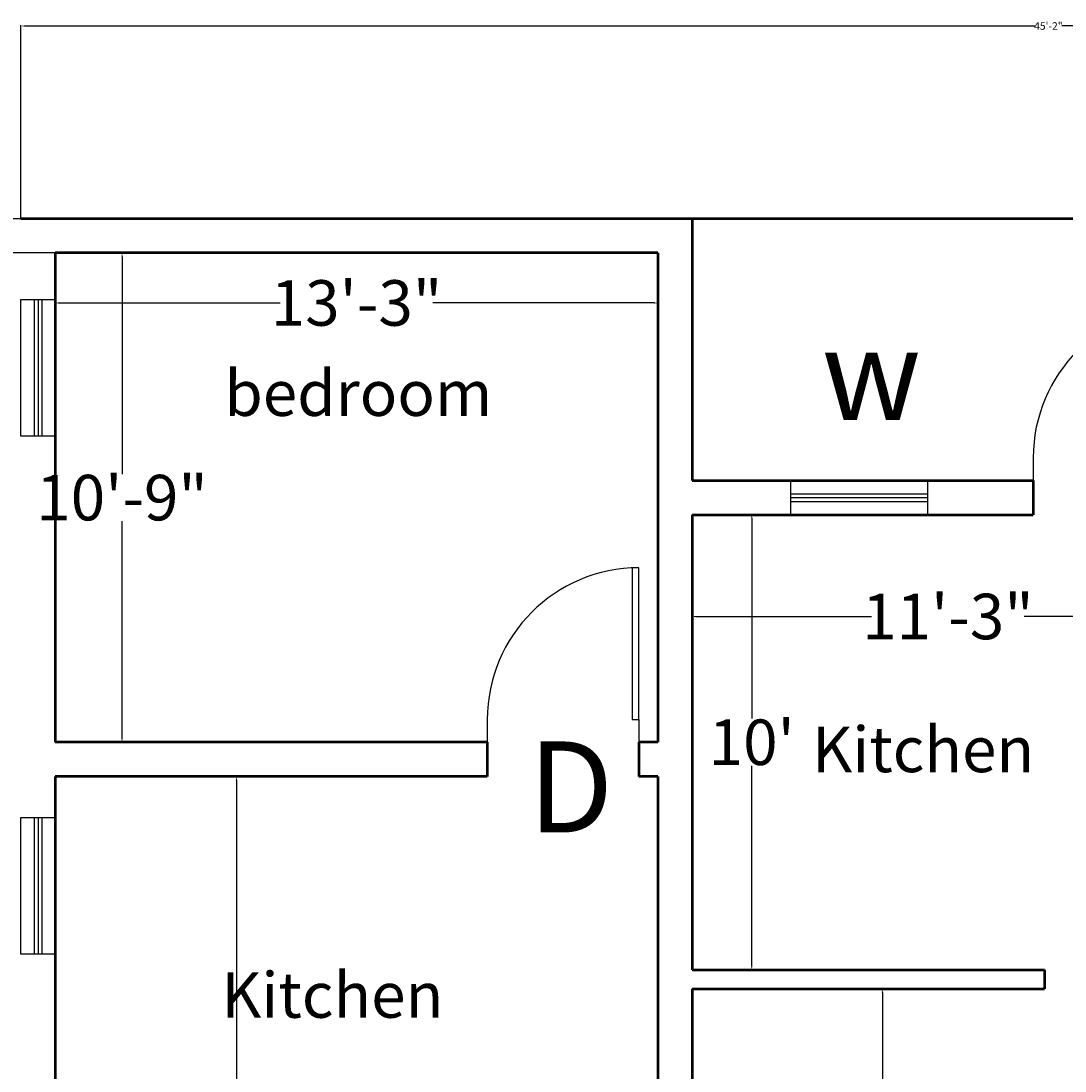
# Model space of a CAD drawing. Units: inches. Extents: x 409 to 7572, y 7 to 725.
# Tile 30 of 38: x 5677 to 5952, y 448 to 725. Entities that reach past the tile are written whole.
import ezdxf

# ---------------------------------------------------------------- set-up
doc = ezdxf.new("R2010")
doc.units = ezdxf.units.IN
doc.header["$MEASUREMENT"] = 0
for name, color, linetype, lineweight in [('A-ANNO-DIMS', 2, 'Continuous', 18), ('A-ANNO-SYMB', 3, 'Continuous', 25), ('A-AREA-IDEN', 7, 'Continuous', 25), ('A-DOOR', 3, 'Continuous', 25), ('A-GLAZ', 4, 'Continuous', 25), ('A-WALL', 7, 'Continuous', 50)]:
    doc.layers.add(name, color=color, linetype=linetype, lineweight=lineweight)
doc.styles.get("Standard").update_dxf_attribs({"font": 'arial.ttf'})
doc.dimstyles.get("Standard").update_dxf_attribs({"dimtxt": 2, "dimasz": 1, "dimexe": 0.18, "dimexo": 0.0625, "dimgap": 0.09, "dimtad": 0, "dimtih": 1, "dimtoh": 1, "dimdec": 0, "dimzin": 0, "dimdsep": 46, "dimlunit": 3, "dimtxsty": 'Standard', "dimcen": 0.09, "dimadec": 0, "dimazin": 0, "dimtfac": 1, "dimtdec": 0, "dimtofl": 0, "dimtmove": 0, "dimatfit": 3, "dimfxl": 1, "dimtolj": 1, "dimtzin": 0, "dimarcsym": 0})

# ---------------------------------------------------------------- blocks, each defined once
blk = doc.blocks.new('*U2')
for p, q in [((0, 0), (0, -6)), ((-40, 0), (-40, -6))]:
    blk.add_line(p, q)
blk.add_lwpolyline([(0, 0), (0, 40), (-1.75, 40), (-1.75, 0)], close=True)
blk.add_arc((0, 0), 40, 90, 180)
blk = doc.blocks.new('*D127')
at = {"layer": 'A-ANNO-DIMS', "color": 0, "lineweight": -2, "transparency": 16777216}
for p, q in [((5685.85, 663.53), (5703.62, 663.53)), ((5703.44, 662.53), (5703.44, 605.25)), ((5703.44, 535.53), (5703.44, 592.81)), ((5685.85, 534.53), (5703.62, 534.53))]:
    blk.add_line(p, q, dxfattribs=at)
at = {"layer": 'A-ANNO-DIMS', "color": 0, "transparency": 16777216}
for points in [[(5703.27, 662.53), (5703.6, 662.53), (5703.44, 663.53)], [(5703.27, 535.53), (5703.6, 535.53), (5703.44, 534.53)]]:
    blk.add_solid(points, dxfattribs=at)
at = {"layer": 'DEFPOINTS', "color": 0, "transparency": 16777216}
for p in [(5685.78, 663.53), (5685.78, 534.53), (5703.44, 534.53)]:
    blk.add_point(p, dxfattribs=at)
at = {"layer": 'A-ANNO-DIMS', "color": 0, "transparency": 16777216, "insert": (5703.44, 599.03), "char_height": 2, "attachment_point": 5}
blk.add_mtext('\\A1;{\\H6x;10\'-9"}', dxfattribs=at)
blk = doc.blocks.new('*D128')
at = {"layer": 'A-ANNO-DIMS', "color": 0, "lineweight": -2, "transparency": 16777216}
for p, q in [((5685.78, 663.47), (5685.78, 650.17)), ((5844.78, 663.47), (5844.78, 650.17)), ((5686.78, 650.35), (5745.15, 650.35)), ((5843.78, 650.35), (5785.42, 650.35))]:
    blk.add_line(p, q, dxfattribs=at)
at = {"layer": 'A-ANNO-DIMS', "color": 0, "transparency": 16777216}
for points in [[(5686.78, 650.52), (5686.78, 650.19), (5685.78, 650.35)], [(5843.78, 650.52), (5843.78, 650.19), (5844.78, 650.35)]]:
    blk.add_solid(points, dxfattribs=at)
at = {"layer": 'DEFPOINTS', "color": 0, "transparency": 16777216}
for p in [(5685.78, 663.53), (5844.78, 663.53), (5844.78, 650.35)]:
    blk.add_point(p, dxfattribs=at)
at = {"layer": 'A-ANNO-DIMS', "color": 0, "transparency": 16777216, "insert": (5765.28, 650.35), "char_height": 2, "attachment_point": 5}
blk.add_mtext('\\A1;{\\H6x;13\'-3"}', dxfattribs=at)
blk = doc.blocks.new('*D137')
at = {"layer": 'A-ANNO-DIMS', "color": 0, "lineweight": -2, "transparency": 16777216}
for p, q in [((5853.85, 594.53), (5869.72, 594.53)), ((5869.54, 593.53), (5869.54, 540.75)), ((5869.54, 475.53), (5869.54, 528.31)), ((5853.85, 474.53), (5869.72, 474.53))]:
    blk.add_line(p, q, dxfattribs=at)
at = {"layer": 'A-ANNO-DIMS', "color": 0, "transparency": 16777216}
for points in [[(5869.37, 593.53), (5869.71, 593.53), (5869.54, 594.53)], [(5869.37, 475.53), (5869.71, 475.53), (5869.54, 474.53)]]:
    blk.add_solid(points, dxfattribs=at)
at = {"layer": 'DEFPOINTS', "color": 0, "transparency": 16777216}
for p in [(5853.78, 594.53), (5853.78, 474.53), (5869.54, 474.53)]:
    blk.add_point(p, dxfattribs=at)
at = {"layer": 'A-ANNO-DIMS', "color": 0, "transparency": 16777216, "insert": (5869.54, 534.53), "char_height": 2, "attachment_point": 5}
blk.add_mtext("\\A1;{\\H6x;10'}", dxfattribs=at)
blk = doc.blocks.new('*D139')
at = {"layer": 'A-ANNO-DIMS', "color": 0, "lineweight": -2, "transparency": 16777216}
for p, q in [((5742.72, 525.53), (5733.44, 525.53)), ((5733.62, 524.53), (5733.62, 428.65)), ((5733.62, 320.53), (5733.62, 416.42)), ((5750.72, 319.53), (5733.44, 319.53))]:
    blk.add_line(p, q, dxfattribs=at)
at = {"layer": 'A-ANNO-DIMS', "color": 0, "transparency": 16777216}
for points in [[(5733.45, 524.53), (5733.79, 524.53), (5733.62, 525.53)], [(5733.45, 320.53), (5733.79, 320.53), (5733.62, 319.53)]]:
    blk.add_solid(points, dxfattribs=at)
at = {"layer": 'DEFPOINTS', "color": 0, "transparency": 16777216}
for p in [(5742.78, 525.53), (5733.62, 319.53), (5750.78, 319.53)]:
    blk.add_point(p, dxfattribs=at)
at = {"layer": 'A-ANNO-DIMS', "color": 0, "transparency": 16777216, "insert": (5733.62, 422.53), "char_height": 2, "attachment_point": 5}
blk.add_mtext('\\A1;{\\H6x;17\'-2"}', dxfattribs=at)
blk = doc.blocks.new('*D135')
at = {"layer": 'A-ANNO-DIMS', "color": 0, "lineweight": -2, "transparency": 16777216}
for p, q in [((5853.78, 563.4), (5853.78, 567.87)), ((5854.78, 567.69), (5901.15, 567.69)), ((5987.78, 567.69), (5941.42, 567.69)), ((5988.78, 563.4), (5988.78, 567.87))]:
    blk.add_line(p, q, dxfattribs=at)
at = {"layer": 'A-ANNO-DIMS', "color": 0, "transparency": 16777216}
for points in [[(5854.78, 567.86), (5854.78, 567.52), (5853.78, 567.69)], [(5987.78, 567.86), (5987.78, 567.52), (5988.78, 567.69)]]:
    blk.add_solid(points, dxfattribs=at)
at = {"layer": 'DEFPOINTS', "color": 0, "transparency": 16777216}
for p in [(5988.78, 567.69), (5853.78, 563.33), (5988.78, 563.33)]:
    blk.add_point(p, dxfattribs=at)
at = {"layer": 'A-ANNO-DIMS', "color": 0, "transparency": 16777216, "insert": (5921.28, 567.69), "char_height": 2, "attachment_point": 5}
blk.add_mtext('\\A1;{\\H6x;11\'-3"}', dxfattribs=at)
blk = doc.blocks.new('*D140')
at = {"layer": 'A-ANNO-DIMS', "color": 0, "lineweight": -2, "transparency": 16777216}
for p, q in [((5908.05, 469.53), (5903.8, 469.53)), ((5903.98, 468.53), (5903.98, 409.65)), ((5903.98, 338.53), (5903.98, 397.42)), ((5909.22, 337.53), (5903.8, 337.53))]:
    blk.add_line(p, q, dxfattribs=at)
at = {"layer": 'A-ANNO-DIMS', "color": 0, "transparency": 16777216}
for points in [[(5903.81, 468.53), (5904.15, 468.53), (5903.98, 469.53)], [(5903.81, 338.53), (5904.15, 338.53), (5903.98, 337.53)]]:
    blk.add_solid(points, dxfattribs=at)
at = {"layer": 'DEFPOINTS', "color": 0, "transparency": 16777216}
for p in [(5908.11, 469.53), (5903.98, 337.53), (5909.28, 337.53)]:
    blk.add_point(p, dxfattribs=at)
at = {"layer": 'A-ANNO-DIMS', "color": 0, "transparency": 16777216, "insert": (5903.98, 403.53), "char_height": 2, "attachment_point": 5}
blk.add_mtext("\\A1;{\\H6x;11'}", dxfattribs=at)
blk = doc.blocks.new('*D146')
at = {"layer": 'A-ANNO-DIMS', "color": 0, "lineweight": -2, "transparency": 16777216}
for p, q in [((5676.78, 672.59), (5676.78, 723.56)), ((5677.78, 723.38), (5944.22, 723.38)), ((6217.78, 723.38), (5951.35, 723.38)), ((6218.78, 672.59), (6218.78, 723.56))]:
    blk.add_line(p, q, dxfattribs=at)
at = {"layer": 'A-ANNO-DIMS', "color": 0, "transparency": 16777216}
for points in [[(5677.78, 723.55), (5677.78, 723.22), (5676.78, 723.38)], [(6217.78, 723.55), (6217.78, 723.22), (6218.78, 723.38)]]:
    blk.add_solid(points, dxfattribs=at)
at = {"layer": 'DEFPOINTS', "color": 0, "transparency": 16777216}
for p in [(5676.78, 723.38), (5676.78, 672.53), (6218.78, 672.53)]:
    blk.add_point(p, dxfattribs=at)
at = {"layer": 'A-ANNO-DIMS', "color": 0, "transparency": 16777216, "insert": (5947.78, 723.38), "char_height": 2, "attachment_point": 5}
blk.add_mtext('\\A1;45\'-2"', dxfattribs=at)
blk = doc.blocks.new('WIN-36')
for p, q in [((1699.82, 514.65), (1699.82, 478.65)), ((1700.82, 514.65), (1700.82, 478.65)), ((1701.82, 514.65), (1701.82, 478.65))]:
    blk.add_line(p, q)
blk.add_lwpolyline([(1705.32, 514.65), (1705.32, 478.65), (1696.32, 478.65), (1696.32, 514.65)], close=True)
blk = doc.blocks.new('*D192')
at = {"layer": 'A-ANNO-DIMS', "color": 0, "lineweight": -2, "transparency": 16777216}
for p, q in [((5676.72, 672.53), (5590.6, 672.53)), ((5590.78, 671.53), (5590.78, 669.14)), ((5590.78, 664.53), (5590.78, 666.92)), ((5685.72, 663.53), (5590.6, 663.53))]:
    blk.add_line(p, q, dxfattribs=at)
at = {"layer": 'A-ANNO-DIMS', "color": 0, "transparency": 16777216}
for points in [[(5590.62, 671.53), (5590.95, 671.53), (5590.78, 672.53)], [(5590.62, 664.53), (5590.95, 664.53), (5590.78, 663.53)]]:
    blk.add_solid(points, dxfattribs=at)
at = {"layer": 'DEFPOINTS', "color": 0, "transparency": 16777216}
for p in [(5676.78, 672.53), (5590.78, 663.53), (5685.78, 663.53)]:
    blk.add_point(p, dxfattribs=at)
at = {"layer": 'A-ANNO-DIMS', "color": 0, "transparency": 16777216, "insert": (5590.78, 668.03), "char_height": 2, "attachment_point": 5}
blk.add_mtext('\\A1;0\'-9"', dxfattribs=at)

msp = doc.modelspace()

# ---------------------------------------------------------------- linework, layer by layer
at = {"layer": 'A-WALL'}
for p, q in [((6218.78, 672.53), (5676.78, 672.53)), ((5853.78, 672.53), (5853.78, 603.53)), ((5844.78, 663.53), (5685.78, 663.53)), ((5685.78, 663.53), (5685.78, 534.53)), ((5844.78, 663.53), (5844.78, 534.53)), ((5844.78, 663.53), (5844.78, 534.53)), ((5853.78, 603.53), (5943.78, 603.53)), ((5943.78, 603.53), (5943.78, 594.53)), ((5853.78, 594.53), (5943.78, 594.53)), ((5853.78, 594.53), (5853.78, 474.53)), ((5799.78, 534.53), (5685.78, 534.53)), ((5799.78, 534.53), (5799.78, 525.53)), ((5844.78, 534.53), (5839.78, 534.53)), ((5839.78, 534.53), (5839.78, 525.53)), ((5799.78, 525.53), (5685.78, 525.53)), ((5685.78, 525.53), (5685.78, 404.53)), ((5844.78, 525.53), (5839.78, 525.53)), ((5844.78, 525.53), (5844.78, 319.53)), ((5853.78, 474.53), (5946.78, 474.53)), ((5946.78, 474.53), (5946.78, 469.53)), ((5853.78, 469.53), (5946.78, 469.53)), ((5853.78, 469.53), (5853.78, 337.53))]:
    msp.add_line(p, q, dxfattribs=at)

# ---------------------------------------------------------------- block references
at = {"layer": 'A-DOOR'}
for p in [(5983.78, 609.53), (5839.78, 540.53)]:
    msp.add_blockref('*U2', p, dxfattribs=at)
at = {"layer": 'A-GLAZ'}
for p in [(3980.46, 136.58), (3980.46, 0)]:
    msp.add_blockref('WIN-36', p, dxfattribs=at)
at = {"layer": 'A-GLAZ', "rotation": 89.99999999999751}
msp.add_blockref('WIN-36', (6394.53, -1101.79), dxfattribs=at)

# ---------------------------------------------------------------- texts
at = {"layer": 'A-ANNO-SYMB', "char_height": 24, "attachment_point": 1}
for s, width, insert in [('w', 18.2582, (5887.96, 643.49)), ('D', 19.1972, (5810.51, 534.75))]:
    msp.add_mtext_dynamic_manual_height_columns(s, width=width, gutter_width=1, heights=[0], dxfattribs=dict(at, insert=insert))
at = {"layer": 'A-AREA-IDEN', "char_height": 12, "attachment_point": 1}
for s, width, insert in [('bedroom', 40.9017, (5730.44, 632.57)), ('Kitchen ', 61.5504, (5885.47, 538.64)), ('Kitchen ', 61.5504, (5729.61, 473.89))]:
    msp.add_mtext_dynamic_manual_height_columns(s, width=width, gutter_width=1, heights=[0], dxfattribs=dict(at, insert=insert))

# ---------------------------------------------------------------- dimensions: what is measured, and where the dimension line sits
at = {"layer": 'A-ANNO-DIMS'}
dim = msp.add_linear_dim(base=(5676.78, 723.38), p1=(6218.78, 672.53), p2=(5676.78, 672.53), dimstyle='Standard', override={"dimclrd": 0, "dimclre": 0, "dimclrt": 0}, dxfattribs=at)
dim.commit()
dim.dimension.update_dxf_attribs({"geometry": '*D146', "text_midpoint": (5947.78, 723.38)})
dim = msp.add_linear_dim(base=(5590.78, 663.53), p1=(5676.78, 672.53), p2=(5685.78, 663.53), angle=90, dimstyle='Standard', override={"dimdec": 1, "dimlfac": 1, "dimrnd": 0, "dimzin": 1, "dimdsep": 46, "dimlunit": 4, "dimfrac": 2}, dxfattribs=at)
dim.commit()
dim.dimension.update_dxf_attribs({"geometry": '*D192', "text_midpoint": (5590.78, 668.03)})
for base, p1, p2, picture, middle in [((5703.44, 534.53), (5685.78, 663.53), (5685.78, 534.53), '*D127', (5703.44, 599.03)), ((5869.54, 474.53), (5853.78, 594.53), (5853.78, 474.53), '*D137', (5869.54, 534.53)), ((5903.98, 337.53), (5908.11, 469.53), (5909.28, 337.53), '*D140', (5903.98, 403.53))]:
    dim = msp.add_linear_dim(base=base, p1=p1, p2=p2, angle=90, text='{\\H6x;<>}', dimstyle='Standard', override={"dimclrd": 0, "dimclre": 0, "dimclrt": 0}, dxfattribs=at)
    dim.commit()
    dim.dimension.update_dxf_attribs({"geometry": picture, "text_midpoint": middle})
for base, p1, p2, picture, middle in [((5844.78, 650.35), (5685.78, 663.53), (5844.78, 663.53), '*D128', (5765.28, 650.35)), ((5988.78, 567.69), (5853.78, 563.33), (5988.78, 563.33), '*D135', (5921.28, 567.69))]:
    dim = msp.add_linear_dim(base=base, p1=p1, p2=p2, text='{\\H6x;<>}', dimstyle='Standard', override={"dimclrd": 0, "dimclre": 0, "dimclrt": 0}, dxfattribs=at)
    dim.commit()
    dim.dimension.update_dxf_attribs({"geometry": picture, "text_midpoint": middle})
dim = msp.add_linear_dim(base=(5733.62, 319.53), p1=(5742.78, 525.53), p2=(5750.78, 319.53), angle=90, text='{\\H6x;<>}', dimstyle='Standard', override={"dimclrd": 0, "dimclre": 0, "dimclrt": 0}, dxfattribs=at)
dim.commit()
dim.dimension.update_dxf_attribs({"geometry": '*D139', "text_midpoint": (5733.62, 422.53), "dimtype": 160})

doc.saveas('drawing.dxf')
